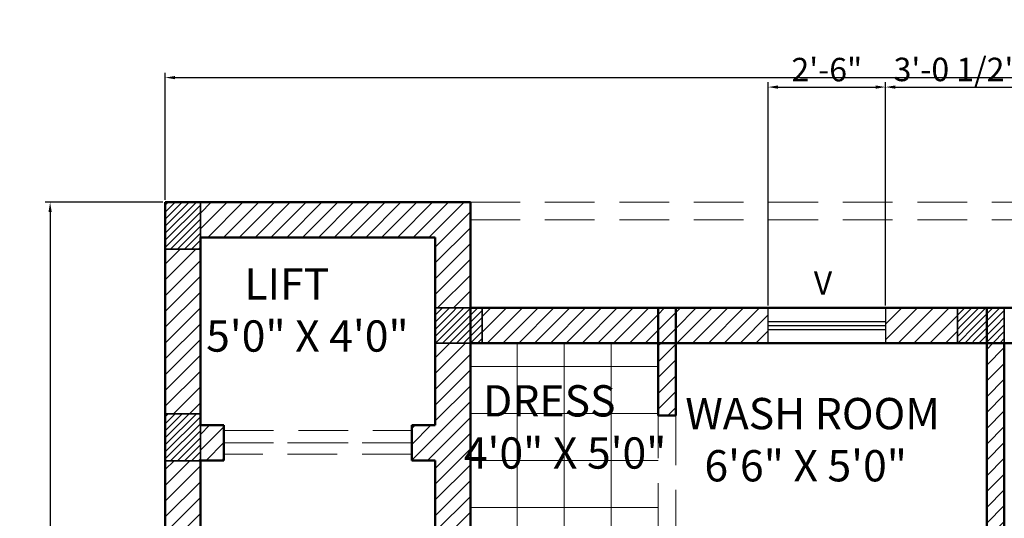
# Model space of a CAD drawing. Units: millimetres. Extents: x 225995 to 227247, y 225507 to 226008.
# Tile 16 of 23: x 226643 to 226894, y 225881 to 226008. Entities that reach past the tile are written whole.
import ezdxf

# ---------------------------------------------------------------- set-up
doc = ezdxf.new("R2010")
doc.units = ezdxf.units.MM
doc.linetypes.add('DASHED', pattern=[19.05, 12.7, -6.35])
for name, color, linetype, lineweight in [('A-ANNO-DIMS', 2, 'Continuous', 18), ('A-ANNO-TEXT', 3, 'Continuous', 18), ('A-AREA-IDEN', 30, 'Continuous', 18), ('A-COLS', 40, 'Continuous', 35), ('A-FLOR-PATT', 8, 'Continuous', 13), ('A-FURN', 9, 'Continuous', 18), ('A-GLAZ', 4, 'Continuous', 25), ('A-WALL', 7, 'Continuous', 50), ('A-WALL-OVHD', 1, 'DASHED', 18), ('A-WALL-PATT', 8, 'Continuous', 13)]:
    doc.layers.add(name, color=color, linetype=linetype, lineweight=lineweight)
doc.styles.get("Standard").update_dxf_attribs({"font": 'arial.ttf'})
doc.dimstyles.new('ISO-25', dxfattribs={"dimtxt": 6, "dimasz": 2.5, "dimexe": 1.25, "dimexo": 0.625, "dimtad": 1, "dimdec": 0, "dimlunit": 3, "dimtxsty": 'Standard', "dimcen": 2.5, "dimadec": 0, "dimazin": 0, "dimtfac": 1, "dimtdec": 0, "dimtmove": 0, "dimatfit": 3, "dimfxl": 1, "dimarcsym": 0})
pattern_1 = [(45, (646.0463, 0.931), (-2.020557627, 2.020557627), [])]
pattern_2 = [(45, (502.0463, 234.931), (-0.898025612, 0.898025612), [])]
pattern_3 = [(45, (368.5463, 234.931), (-0.898025612, 0.898025612), [])]

# ---------------------------------------------------------------- blocks, each defined once
blk = doc.blocks.new('*D70')
at = {"layer": 'A-ANNO-DIMS', "color": 0, "lineweight": -2, "transparency": 16777216}
for p, q in [((226679.92, 225962.33), (226679.92, 225994.83)), ((226682.42, 225993.58), (227209.42, 225993.58)), ((227211.92, 225962.33), (227211.92, 225994.83))]:
    blk.add_line(p, q, dxfattribs=at)
at = {"layer": 'A-ANNO-DIMS', "color": 0, "transparency": 16777216}
for points in [[(226682.42, 225993.99), (226682.42, 225993.16), (226679.92, 225993.58)], [(227209.42, 225993.99), (227209.42, 225993.16), (227211.92, 225993.58)]]:
    blk.add_solid(points, dxfattribs=at)
at = {"layer": 'Defpoints', "color": 0, "transparency": 16777216}
for p in [(227211.92, 225993.58), (226679.92, 225961.7), (227211.92, 225961.7)]:
    blk.add_point(p, dxfattribs=at)
at = {"layer": 'A-ANNO-DIMS', "color": 0, "transparency": 16777216, "insert": (226945.92, 226000.2), "char_height": 12, "attachment_point": 5}
blk.add_mtext('44\'-4"', dxfattribs=at)
blk = doc.blocks.new('*D113')
at = {"layer": 'A-ANNO-DIMS', "color": 0, "lineweight": -2, "transparency": 16777216}
for p, q in [((226679.3, 225961.7), (226649.22, 225961.7)), ((226650.47, 225959.2), (226650.47, 225553.2)), ((226679.3, 225550.7), (226649.22, 225550.7))]:
    blk.add_line(p, q, dxfattribs=at)
at = {"layer": 'A-ANNO-DIMS', "color": 0, "transparency": 16777216}
for points in [[(226650.06, 225959.2), (226650.89, 225959.2), (226650.47, 225961.7)], [(226650.06, 225553.2), (226650.89, 225553.2), (226650.47, 225550.7)]]:
    blk.add_solid(points, dxfattribs=at)
at = {"layer": 'Defpoints', "color": 0, "transparency": 16777216}
for p in [(226679.92, 225961.7), (226650.47, 225550.7), (226679.92, 225550.7)]:
    blk.add_point(p, dxfattribs=at)
at = {"layer": 'A-ANNO-DIMS', "color": 0, "transparency": 16777216, "insert": (226646.78, 225756.2), "char_height": 6, "attachment_point": 5, "rotation": 90}
blk.add_mtext('34\'-3"', dxfattribs=at)
blk = doc.blocks.new('*D116')
at = {"layer": 'A-ANNO-DIMS', "color": 0, "lineweight": -2, "transparency": 16777216}
for p, q in [((226834.05, 225935.33), (226834.05, 225992.4)), ((226864.05, 225935.33), (226864.05, 225992.4)), ((226836.55, 225991.15), (226861.55, 225991.15))]:
    blk.add_line(p, q, dxfattribs=at)
at = {"layer": 'A-ANNO-DIMS', "color": 0, "transparency": 16777216}
for points in [[(226836.55, 225991.57), (226836.55, 225990.74), (226834.05, 225991.15)], [(226861.55, 225991.57), (226861.55, 225990.74), (226864.05, 225991.15)]]:
    blk.add_solid(points, dxfattribs=at)
at = {"layer": 'Defpoints', "color": 0, "transparency": 16777216}
for p in [(226864.05, 225991.15), (226834.05, 225934.7), (226864.05, 225934.7)]:
    blk.add_point(p, dxfattribs=at)
at = {"layer": 'A-ANNO-DIMS', "color": 0, "transparency": 16777216, "insert": (226849.05, 225994.84), "char_height": 6, "attachment_point": 5}
blk.add_mtext('2\'-6"', dxfattribs=at)
blk = doc.blocks.new('*D117')
at = {"layer": 'A-ANNO-DIMS', "color": 0, "lineweight": -2, "transparency": 16777216}
for p, q in [((226864.05, 225935.33), (226864.05, 225992.4)), ((226900.42, 225935.33), (226900.42, 225992.4)), ((226866.55, 225991.15), (226897.92, 225991.15))]:
    blk.add_line(p, q, dxfattribs=at)
at = {"layer": 'A-ANNO-DIMS', "color": 0, "transparency": 16777216}
for points in [[(226866.55, 225991.57), (226866.55, 225990.74), (226864.05, 225991.15)], [(226897.92, 225991.57), (226897.92, 225990.74), (226900.42, 225991.15)]]:
    blk.add_solid(points, dxfattribs=at)
at = {"layer": 'Defpoints', "color": 0, "transparency": 16777216}
for p in [(226900.42, 225991.15), (226864.05, 225934.7), (226900.42, 225934.7)]:
    blk.add_point(p, dxfattribs=at)
at = {"layer": 'A-ANNO-DIMS', "color": 0, "transparency": 16777216, "insert": (226882.23, 225994.88), "char_height": 6, "attachment_point": 5}
blk.add_mtext('3\'-0 1/2"', dxfattribs=at)

msp = doc.modelspace()

# ---------------------------------------------------------------- hatches: boundary and pattern name
at = {"layer": 'A-WALL-PATT'}
h = msp.add_hatch(dxfattribs=at)
h.set_pattern_fill('ANSI31', color=256, scale=0.4)
h.set_pattern_definition([(45, (577.0463, 378.931), (-0.898025612, 0.898025612), [])])
h.paths.add_polyline_path([(226688.92, 225961.7), (226679.92, 225961.7), (226679.92, 225949.7), (226688.92, 225949.7)])
h = msp.add_hatch(dxfattribs=at)
h.set_pattern_fill('ANSI31', color=256, scale=0.9)
h.set_pattern_definition(pattern_1)
h.paths.add_polyline_path([(226757.92, 225961.7), (226688.92, 225961.7), (226688.92, 225952.7), (226748.92, 225952.7), (226748.92, 225934.7), (226757.92, 225934.7)])
h = msp.add_hatch(dxfattribs=at)
h.set_pattern_fill('ANSI31', color=256, scale=0.9)
h.set_pattern_definition(pattern_1)
h.paths.add_polyline_path([(226688.92, 225949.7), (226679.92, 225949.7), (226679.92, 225907.61), (226688.92, 225907.61)])
h = msp.add_hatch(dxfattribs=at)
h.set_pattern_fill('ANSI31', color=256, scale=0.4)
h.set_pattern_definition(pattern_3)
h.paths.add_polyline_path([(226753.42, 225934.7), (226748.92, 225934.7), (226748.92, 225930.2), (226753.42, 225930.2)])
h = msp.add_hatch(dxfattribs=at)
h.set_pattern_fill('ANSI31', color=256, scale=0.4)
h.set_pattern_definition(pattern_3)
h.paths.add_polyline_path([(226760.92, 225934.7), (226753.42, 225934.7), (226753.42, 225930.2), (226760.92, 225930.2)])
h = msp.add_hatch(dxfattribs=at)
h.set_pattern_fill('ANSI31', color=256, scale=0.9)
h.paths.add_polyline_path([(226805.92, 225934.7), (226760.92, 225934.7), (226760.92, 225925.7), (226805.92, 225925.7)])
h = msp.add_hatch(dxfattribs=at)
h.set_pattern_fill('ANSI31', color=256, scale=0.9)
h.paths.add_polyline_path([(226810.42, 225934.7), (226805.92, 225934.7), (226805.92, 225925.7), (226810.42, 225925.7)])
h = msp.add_hatch(dxfattribs=at)
h.set_pattern_fill('ANSI31', color=256, scale=0.9)
h.paths.add_polyline_path([(226834.05, 225934.7), (226810.42, 225934.7), (226810.42, 225925.7), (226834.05, 225925.7)])
h = msp.add_hatch(dxfattribs=at)
h.set_pattern_fill('ANSI31', color=256, scale=0.9)
h.paths.add_polyline_path([(226882.42, 225934.7), (226864.05, 225934.7), (226864.05, 225925.7), (226882.42, 225925.7)])
h = msp.add_hatch(dxfattribs=at)
h.set_pattern_fill('ANSI31', color=256, scale=0.4)
h.set_pattern_definition(pattern_2)
h.paths.add_polyline_path([(226886.92, 225934.7), (226882.42, 225934.7), (226882.42, 225930.2), (226886.92, 225930.2)])
h = msp.add_hatch(dxfattribs=at)
h.set_pattern_fill('ANSI31', color=256, scale=0.4)
h.set_pattern_definition(pattern_2)
h.paths.add_polyline_path([(226894.42, 225934.7), (226886.92, 225934.7), (226886.92, 225930.2), (226894.42, 225930.2)])
h = msp.add_hatch(dxfattribs=at)
h.set_pattern_fill('ANSI31', color=256, scale=0.4)
h.set_pattern_definition(pattern_3)
h.paths.add_polyline_path([(226753.42, 225930.2), (226748.92, 225930.2), (226748.92, 225925.7), (226753.42, 225925.7)])
h = msp.add_hatch(dxfattribs=at)
h.set_pattern_fill('ANSI31', color=256, scale=0.4)
h.set_pattern_definition(pattern_3)
h.paths.add_polyline_path([(226760.92, 225930.2), (226753.42, 225930.2), (226753.42, 225925.7), (226760.92, 225925.7)])
h = msp.add_hatch(dxfattribs=at)
h.set_pattern_fill('ANSI31', color=256, scale=0.4)
h.set_pattern_definition(pattern_2)
h.paths.add_polyline_path([(226886.92, 225930.2), (226882.42, 225930.2), (226882.42, 225925.7), (226886.92, 225925.7)])
h = msp.add_hatch(dxfattribs=at)
h.set_pattern_fill('ANSI31', color=256, scale=0.4)
h.set_pattern_definition(pattern_2)
h.paths.add_polyline_path([(226894.42, 225930.2), (226886.92, 225930.2), (226886.92, 225925.7), (226894.42, 225925.7)])
h = msp.add_hatch(dxfattribs=at)
h.set_pattern_fill('ANSI31', color=256, scale=0.9)
h.set_pattern_definition(pattern_1)
h.paths.add_polyline_path([(226757.92, 225925.7), (226748.92, 225925.7), (226748.92, 225904.7), (226742.92, 225904.7), (226742.92, 225895.7), (226748.92, 225895.7), (226748.92, 225821.85), (226757.92, 225821.85)])
h = msp.add_hatch(dxfattribs=at)
h.set_pattern_fill('ANSI31', color=256, scale=0.9)
h.paths.add_polyline_path([(226810.42, 225925.7), (226805.92, 225925.7), (226805.92, 225907.21), (226810.42, 225907.21)])
h = msp.add_hatch(dxfattribs=at)
h.set_pattern_fill('ANSI31', color=256, scale=0.9)
h.paths.add_polyline_path([(226894.42, 225925.7), (226889.92, 225925.7), (226889.92, 225818.84), (226894.42, 225818.84)])
h = msp.add_hatch(dxfattribs=at)
h.set_pattern_fill('ANSI31', color=256, scale=0.4)
h.set_pattern_definition([(45, (577.0463, 324.8396), (-0.898025612, 0.898025612), [])])
h.paths.add_polyline_path([(226688.92, 225907.61), (226679.92, 225907.61), (226679.92, 225895.61), (226688.92, 225895.61)])
h = msp.add_hatch(dxfattribs=at)
h.set_pattern_fill('ANSI31', color=256, scale=0.9)
h.set_pattern_definition(pattern_1)
h.paths.add_polyline_path([(226694.92, 225904.7), (226688.92, 225904.7), (226688.92, 225895.7), (226694.92, 225895.7)])
h = msp.add_hatch(dxfattribs=at)
h.set_pattern_fill('ANSI31', color=256, scale=0.9)
h.set_pattern_definition(pattern_1)
h.paths.add_polyline_path([(226688.92, 225895.61), (226679.92, 225895.61), (226679.92, 225709.35), (226688.92, 225709.35)])

# ---------------------------------------------------------------- linework, layer by layer
at = {"layer": 'A-COLS'}
for points in [[(226688.92, 225949.7), (226679.92, 225949.7), (226679.92, 225961.7), (226688.92, 225961.7)], [(226748.92, 225925.7), (226748.92, 225934.7), (226760.92, 225934.7), (226760.92, 225925.7)], [(226882.42, 225925.7), (226882.42, 225934.7), (226894.42, 225934.7), (226894.42, 225925.7)], [(226688.92, 225895.61), (226679.92, 225895.61), (226679.92, 225907.61), (226688.92, 225907.61)]]:
    msp.add_lwpolyline(points, close=True, dxfattribs=at)
at = {"layer": 'A-FLOR-PATT'}
for p, q in [((226769.92, 225700.7), (226769.92, 225925.7)), ((226781.92, 225700.7), (226781.92, 225925.7)), ((226793.92, 225700.7), (226793.92, 225925.7)), ((226757.92, 225919.7), (226805.92, 225919.7)), ((226757.92, 225907.7), (226805.92, 225907.7)), ((226757.92, 225895.7), (226805.92, 225895.7)), ((226757.92, 225883.7), (226805.92, 225883.7))]:
    msp.add_line(p, q, dxfattribs=at)
at = {"layer": 'A-FURN'}
for p, q in [((226834.05, 225934.7), (226834.05, 225925.7)), ((226864.05, 225934.7), (226864.05, 225925.7))]:
    msp.add_line(p, q, dxfattribs=at)
at = {"layer": 'A-GLAZ'}
for p, q in [((226834.05, 225931.2), (226864.05, 225931.2)), ((226834.05, 225930.2), (226864.05, 225930.2)), ((226834.05, 225929.2), (226864.05, 225929.2))]:
    msp.add_line(p, q, dxfattribs=at)
msp.add_lwpolyline([(226834.05, 225934.7), (226864.05, 225934.7), (226864.05, 225925.7), (226834.05, 225925.7)], close=True, dxfattribs=at)
at = {"layer": 'A-WALL'}
for p, q in [((226679.92, 225673.7), (226679.92, 225961.7)), ((226757.92, 225961.7), (226679.92, 225961.7)), ((226679.92, 225961.7), (226757.92, 225961.7)), ((226679.92, 225673.7), (226679.92, 225961.7)), ((226757.92, 225810.2), (226757.92, 225961.7)), ((226757.92, 225961.7), (226757.92, 225934.7)), ((226688.92, 225952.7), (226748.92, 225952.7)), ((226688.92, 225904.7), (226688.92, 225952.7)), ((226748.92, 225952.7), (226688.92, 225952.7)), ((226688.92, 225952.7), (226688.92, 225904.7)), ((226748.92, 225904.7), (226748.92, 225952.7)), ((226748.92, 225904.7), (226748.92, 225952.7)), ((226757.92, 225934.7), (227211.92, 225934.7)), ((226757.92, 225934.7), (227211.92, 225934.7)), ((226805.92, 225907.21), (226805.92, 225934.7)), ((226810.42, 225907.21), (226810.42, 225934.7)), ((226889.92, 225741.2), (226889.92, 225934.7)), ((226757.92, 225925.7), (227026.42, 225925.7)), ((226805.92, 225925.7), (226757.92, 225925.7)), ((226757.92, 225925.7), (226757.92, 225865.7)), ((226805.92, 225907.21), (226805.92, 225925.7)), ((226889.92, 225925.7), (226810.42, 225925.7)), ((226810.42, 225925.7), (226810.42, 225907.21)), ((226889.92, 225741.2), (226889.92, 225925.7)), ((227026.42, 225925.7), (226894.42, 225925.7)), ((226894.42, 225925.7), (226894.42, 225741.2)), ((226805.92, 225907.21), (226810.42, 225907.21)), ((226810.42, 225907.21), (226805.92, 225907.21)), ((226688.92, 225904.7), (226694.92, 225904.7)), ((226688.92, 225904.7), (226694.92, 225904.7)), ((226694.92, 225904.7), (226694.92, 225895.7)), ((226694.92, 225904.7), (226694.92, 225895.7)), ((226742.92, 225904.7), (226748.92, 225904.7)), ((226742.92, 225904.7), (226742.92, 225895.7)), ((226742.92, 225895.7), (226742.92, 225904.7)), ((226742.92, 225904.7), (226748.92, 225904.7)), ((226889.92, 225906.2), (226890.09, 225906.2)), ((226688.92, 225895.7), (226694.92, 225895.7)), ((226688.92, 225673.7), (226688.92, 225895.7)), ((226694.92, 225895.7), (226688.92, 225895.61)), ((226688.92, 225895.61), (226688.92, 225673.7)), ((226742.92, 225895.7), (226748.92, 225895.7)), ((226748.92, 225895.7), (226742.92, 225895.7)), ((226748.92, 225691.7), (226748.92, 225895.7)), ((226748.92, 225691.7), (226748.92, 225895.7))]:
    msp.add_line(p, q, dxfattribs=at)
at = {"layer": 'A-WALL-OVHD'}
for p, q in [((226757.92, 225961.7), (227211.92, 225961.7)), ((226757.92, 225957.2), (227207.42, 225957.2))]:
    msp.add_line(p, q, dxfattribs=at)
for points in [[(226805.92, 225907.21), (226810.42, 225907.21), (226810.42, 225877.21), (226805.92, 225877.21)], [(226694.92, 225903.34), (226742.92, 225903.34), (226742.92, 225897.27), (226694.92, 225897.27)], [(226694.92, 225900.2), (226742.92, 225900.2), (226742.92, 225900.2), (226694.92, 225900.2)]]:
    msp.add_lwpolyline(points, close=True, dxfattribs=at)

# ---------------------------------------------------------------- texts
at = {"layer": 'A-ANNO-TEXT', "insert": (226840.2, 225944.08), "char_height": 6, "attachment_point": 1}
msp.add_mtext_dynamic_manual_height_columns('   V', width=24.8115, gutter_width=12.5, heights=[0], dxfattribs=at)
at = {"layer": 'A-AREA-IDEN', "char_height": 8, "attachment_point": 1}
for s, insert in [('       LIFT\\P   5\'0" X 4\'0"', (226683.03, 225944.84)), ('     DRESS\\P   4\'0" X 5\'0"', (226748.92, 225914.93)), (' WASH ROOM\\P   6\'6" X 5\'0"', (226810.42, 225911.67))]:
    msp.add_mtext_dynamic_manual_height_columns(s, width=85.4795, gutter_width=12.5, heights=[0], dxfattribs=dict(at, insert=insert))

# ---------------------------------------------------------------- dimensions: what is measured, and where the dimension line sits
at = {"layer": 'A-ANNO-DIMS'}
for base, p1, p2, override, picture, middle in [((227211.92, 225993.58), (226679.92, 225961.7), (227211.92, 225961.7), {"dimtxt": 12, "dimclrd": 0, "dimclre": 0, "dimclrt": 0}, '*D70', (226945.92, 226000.2)), ((226900.42, 225991.15), (226864.05, 225934.7), (226900.42, 225934.7), {"dimdec": 1, "dimlfac": 1, "dimrnd": 0, "dimzin": 1, "dimdsep": 46, "dimlunit": 4, "dimfrac": 2}, '*D117', (226882.23, 225994.88)), ((226864.05, 225991.15), (226834.05, 225934.7), (226864.05, 225934.7), {"dimdec": 1, "dimlfac": 1, "dimrnd": 0, "dimzin": 1, "dimdsep": 46, "dimlunit": 4, "dimfrac": 2}, '*D116', (226849.05, 225994.84))]:
    dim = msp.add_linear_dim(base=base, p1=p1, p2=p2, dimstyle='ISO-25', override=override, dxfattribs=at)
    dim.commit()
    dim.dimension.update_dxf_attribs({"geometry": picture, "text_midpoint": middle})
dim = msp.add_linear_dim(base=(226650.47, 225550.7), p1=(226679.92, 225961.7), p2=(226679.92, 225550.7), angle=90, dimstyle='ISO-25', override={"dimdec": 1, "dimlfac": 1, "dimrnd": 0, "dimzin": 1, "dimdsep": 46, "dimlunit": 4, "dimfrac": 2}, dxfattribs=at)
dim.commit()
dim.dimension.update_dxf_attribs({"geometry": '*D113', "text_midpoint": (226646.78, 225756.2)})

doc.saveas('drawing.dxf')
